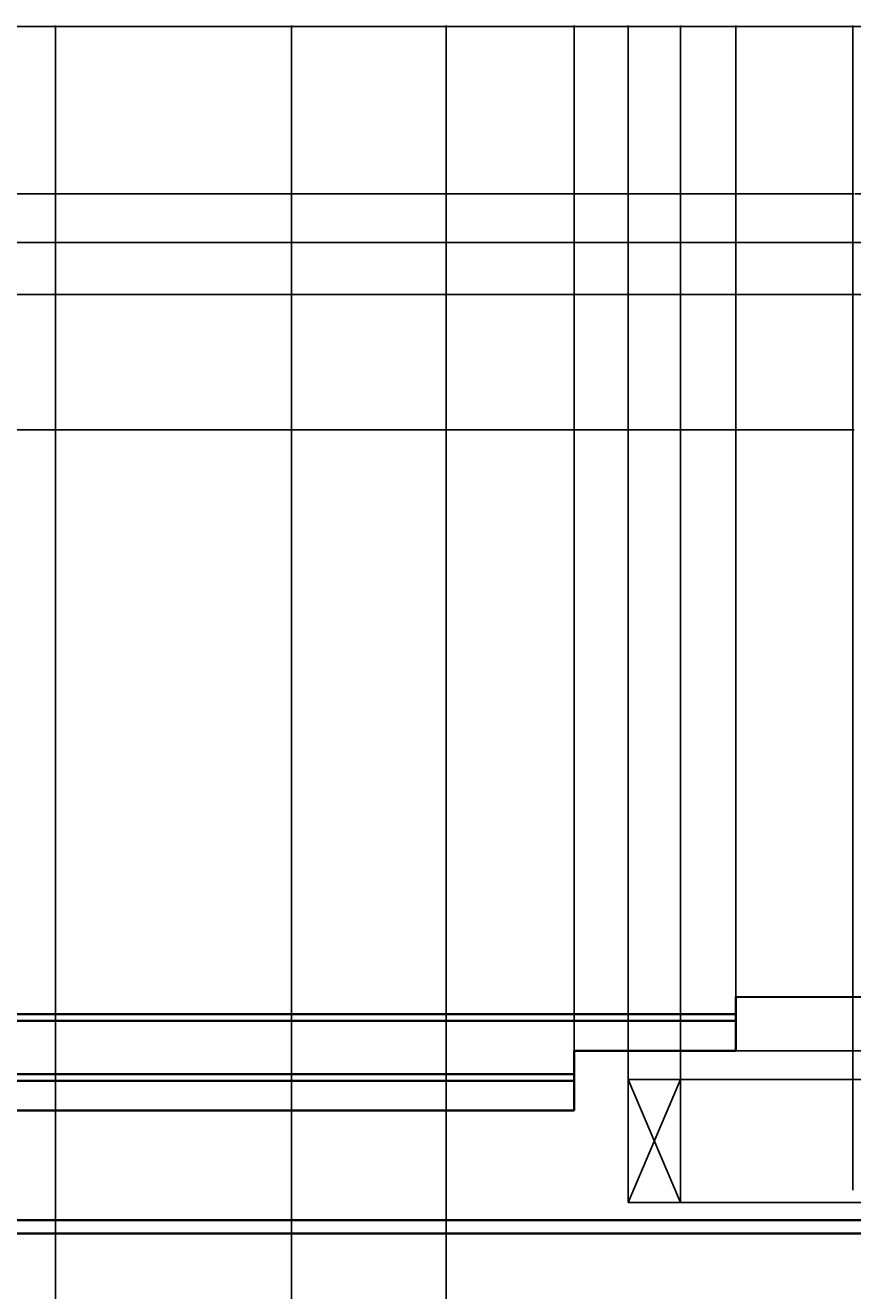
# Model space of a CAD drawing. Units: inches. Extents: x 93 to 565, y 123 to 656.
# Tile 13 of 18: x 291 to 418, y 463 to 656. Entities that reach past the tile are written whole.
import ezdxf

# ---------------------------------------------------------------- set-up
doc = ezdxf.new("R2010")
doc.units = ezdxf.units.IN
doc.header["$MEASUREMENT"] = 0
for name, color, linetype, lineweight in [('A-ANNO-DIMS', 2, 'Continuous', 18), ('A-ELEV', 7, 'Continuous', 35), ('A-GLAZ', 4, 'Continuous', 25)]:
    doc.layers.add(name, color=color, linetype=linetype, lineweight=lineweight)
doc.styles.get("Standard").update_dxf_attribs({"font": 'arial.ttf'})
doc.dimstyles.get("Standard").update_dxf_attribs({"dimtxt": 0.18, "dimasz": 0.18, "dimexe": 0.18, "dimexo": 0.0625, "dimgap": 0.09, "dimtad": 0, "dimtih": 1, "dimtoh": 1, "dimdec": 4, "dimzin": 0, "dimdsep": 46, "dimtxsty": 'Standard', "dimcen": 0.09, "dimadec": 0, "dimazin": 0, "dimtfac": 1, "dimtdec": 4, "dimtofl": 0, "dimtmove": 0, "dimatfit": 3, "dimfxl": 1, "dimtolj": 1, "dimtzin": 0, "dimarcsym": 0})

# ---------------------------------------------------------------- blocks, each defined once
blk = doc.blocks.new('*U9')
for p, q in [((0, 0), (38, 89)), ((38, 0), (0, 89))]:
    blk.add_line(p, q)
blk.add_lwpolyline([(0, 0), (38, 0), (38, 89), (0, 89)], close=True)
blk = doc.blocks.new('*D26')
at = {"layer": 'A-ANNO-DIMS', "color": 0, "lineweight": -2, "transparency": 16777216}
for p, q in [((119.08, 519.16), (119.08, 656.13)), ((119.26, 655.95), (328.79, 655.95)), ((538.9, 655.95), (329.37, 655.95)), ((539.08, 630.47), (539.08, 656.13))]:
    blk.add_line(p, q, dxfattribs=at)
at = {"layer": 'A-ANNO-DIMS', "color": 0, "transparency": 16777216}
for points in [[(119.26, 655.98), (119.26, 655.92), (119.08, 655.95)], [(538.9, 655.98), (538.9, 655.92), (539.08, 655.95)]]:
    blk.add_solid(points, dxfattribs=at)
at = {"layer": 'Defpoints', "color": 0, "transparency": 16777216}
for p in [(539.08, 655.95), (539.08, 630.4), (119.08, 519.1)]:
    blk.add_point(p, dxfattribs=at)
at = {"layer": 'A-ANNO-DIMS', "color": 0, "transparency": 16777216, "insert": (329.08, 655.95), "char_height": 0.18, "attachment_point": 5}
blk.add_mtext('\\A1;420', dxfattribs=at)
blk = doc.blocks.new('*D28')
at = {"layer": 'A-ANNO-DIMS', "color": 0, "lineweight": -2, "transparency": 16777216}
for p, q in [((210.54, 519.04), (210.54, 134)), ((295.69, 183.67), (295.69, 134)), ((210.72, 134.18), (252.72, 134.18)), ((295.51, 134.18), (253.51, 134.18))]:
    blk.add_line(p, q, dxfattribs=at)
at = {"layer": 'A-ANNO-DIMS', "color": 0, "transparency": 16777216}
for points in [[(210.72, 134.21), (210.72, 134.15), (210.54, 134.18)], [(295.51, 134.21), (295.51, 134.15), (295.69, 134.18)]]:
    blk.add_solid(points, dxfattribs=at)
at = {"layer": 'Defpoints', "color": 0, "transparency": 16777216}
for p in [(210.54, 519.1), (295.69, 183.73), (295.69, 134.18)]:
    blk.add_point(p, dxfattribs=at)
at = {"layer": 'A-ANNO-DIMS', "color": 0, "transparency": 16777216, "insert": (253.12, 134.18), "char_height": 0.18, "attachment_point": 5}
blk.add_mtext('\\A1;85.14', dxfattribs=at)
blk = doc.blocks.new('*D29')
at = {"layer": 'A-ANNO-DIMS', "color": 0, "lineweight": -2, "transparency": 16777216}
for p, q in [((437.19, 594.34), (437.19, 134)), ((295.69, 183.67), (295.69, 134)), ((295.87, 134.18), (366.05, 134.18)), ((437.01, 134.18), (366.82, 134.18))]:
    blk.add_line(p, q, dxfattribs=at)
at = {"layer": 'A-ANNO-DIMS', "color": 0, "transparency": 16777216}
for points in [[(295.87, 134.21), (295.87, 134.15), (295.69, 134.18)], [(437.01, 134.21), (437.01, 134.15), (437.19, 134.18)]]:
    blk.add_solid(points, dxfattribs=at)
at = {"layer": 'Defpoints', "color": 0, "transparency": 16777216}
for p in [(437.19, 594.4), (295.69, 183.73), (437.19, 134.18)]:
    blk.add_point(p, dxfattribs=at)
at = {"layer": 'A-ANNO-DIMS', "color": 0, "transparency": 16777216, "insert": (366.44, 134.18), "char_height": 0.18, "attachment_point": 5}
blk.add_mtext('\\A1;141.5', dxfattribs=at)
blk = doc.blocks.new('*D31')
at = {"layer": 'A-ANNO-DIMS', "color": 0, "lineweight": -2, "transparency": 16777216}
for p, q in [((417.87, 630.4), (564.81, 630.4)), ((564.63, 630.22), (564.63, 395.25)), ((564.63, 159.91), (564.63, 394.89)), ((119.14, 159.73), (564.81, 159.73))]:
    blk.add_line(p, q, dxfattribs=at)
at = {"layer": 'A-ANNO-DIMS', "color": 0, "transparency": 16777216}
for points in [[(564.6, 630.22), (564.66, 630.22), (564.63, 630.4)], [(564.6, 159.91), (564.66, 159.91), (564.63, 159.73)]]:
    blk.add_solid(points, dxfattribs=at)
at = {"layer": 'Defpoints', "color": 0, "transparency": 16777216}
for p in [(417.81, 630.4), (564.63, 630.4), (119.08, 159.73)]:
    blk.add_point(p, dxfattribs=at)
at = {"layer": 'A-ANNO-DIMS', "color": 0, "transparency": 16777216, "insert": (564.63, 395.07), "char_height": 0.18, "attachment_point": 5}
blk.add_mtext('\\A1;470.7', dxfattribs=at)
blk = doc.blocks.new('*D36')
at = {"layer": 'A-ANNO-DIMS', "color": 0, "lineweight": -2, "transparency": 16777216}
for p, q in [((417.75, 594.4), (93.35, 594.4)), ((93.53, 594.22), (93.53, 556.93)), ((93.53, 519.28), (93.53, 556.57)), ((119.02, 519.1), (93.35, 519.1))]:
    blk.add_line(p, q, dxfattribs=at)
at = {"layer": 'A-ANNO-DIMS', "color": 0, "transparency": 16777216}
for points in [[(93.5, 594.22), (93.56, 594.22), (93.53, 594.4)], [(93.5, 519.28), (93.56, 519.28), (93.53, 519.1)]]:
    blk.add_solid(points, dxfattribs=at)
at = {"layer": 'Defpoints', "color": 0, "transparency": 16777216}
for p in [(93.53, 594.4), (417.81, 594.4), (119.08, 519.1)]:
    blk.add_point(p, dxfattribs=at)
at = {"layer": 'A-ANNO-DIMS', "color": 0, "transparency": 16777216, "insert": (93.53, 556.75), "char_height": 0.18, "attachment_point": 5}
blk.add_mtext('\\A1;75.3', dxfattribs=at)
blk = doc.blocks.new('*D66')
at = {"layer": 'A-ANNO-DIMS', "color": 0, "lineweight": -2, "transparency": 16777216}
for p, q in [((295.81, 420.63), (295.81, 656.13)), ((295.99, 655.95), (313.59, 655.95)), ((331.63, 655.95), (314.03, 655.95)), ((331.81, 420.63), (331.81, 656.13))]:
    blk.add_line(p, q, dxfattribs=at)
at = {"layer": 'A-ANNO-DIMS', "color": 0, "transparency": 16777216}
for points in [[(295.99, 655.98), (295.99, 655.92), (295.81, 655.95)], [(331.63, 655.98), (331.63, 655.92), (331.81, 655.95)]]:
    blk.add_solid(points, dxfattribs=at)
at = {"layer": 'Defpoints', "color": 0, "transparency": 16777216}
for p in [(331.81, 655.95), (295.81, 420.57), (331.81, 420.57)]:
    blk.add_point(p, dxfattribs=at)
at = {"layer": 'A-ANNO-DIMS', "color": 0, "transparency": 16777216, "insert": (313.81, 655.95), "char_height": 0.18, "attachment_point": 5}
blk.add_mtext('\\A1;36', dxfattribs=at)
blk = doc.blocks.new('*D68')
at = {"layer": 'A-ANNO-DIMS', "color": 0, "lineweight": -2, "transparency": 16777216}
for p, q in [((331.81, 420.63), (331.81, 656.13)), ((331.99, 655.95), (343.24, 655.95)), ((355.28, 655.95), (344.03, 655.95)), ((355.46, 420.63), (355.46, 656.13))]:
    blk.add_line(p, q, dxfattribs=at)
at = {"layer": 'A-ANNO-DIMS', "color": 0, "transparency": 16777216}
for points in [[(331.99, 655.98), (331.99, 655.92), (331.81, 655.95)], [(355.28, 655.98), (355.28, 655.92), (355.46, 655.95)]]:
    blk.add_solid(points, dxfattribs=at)
at = {"layer": 'Defpoints', "color": 0, "transparency": 16777216}
for p in [(355.46, 655.95), (331.81, 420.57), (355.46, 420.57)]:
    blk.add_point(p, dxfattribs=at)
at = {"layer": 'A-ANNO-DIMS', "color": 0, "transparency": 16777216, "insert": (343.64, 655.95), "char_height": 0.18, "attachment_point": 5}
blk.add_mtext('\\A1;23.65', dxfattribs=at)
blk = doc.blocks.new('*D69')
at = {"layer": 'A-ANNO-DIMS', "color": 0, "lineweight": -2, "transparency": 16777216}
for p, q in [((355.46, 420.63), (355.46, 656.13)), ((355.64, 655.95), (391.65, 655.95)), ((428.44, 655.95), (392.43, 655.95)), ((428.62, 420.63), (428.62, 656.13))]:
    blk.add_line(p, q, dxfattribs=at)
at = {"layer": 'A-ANNO-DIMS', "color": 0, "transparency": 16777216}
for points in [[(355.64, 655.98), (355.64, 655.92), (355.46, 655.95)], [(428.44, 655.98), (428.44, 655.92), (428.62, 655.95)]]:
    blk.add_solid(points, dxfattribs=at)
at = {"layer": 'Defpoints', "color": 0, "transparency": 16777216}
for p in [(428.62, 655.95), (355.46, 420.57), (428.62, 420.57)]:
    blk.add_point(p, dxfattribs=at)
at = {"layer": 'A-ANNO-DIMS', "color": 0, "transparency": 16777216, "insert": (392.04, 655.95), "char_height": 0.18, "attachment_point": 5}
blk.add_mtext('\\A1;73.16', dxfattribs=at)
blk = doc.blocks.new('*D75')
at = {"layer": 'A-ANNO-DIMS', "color": 0, "lineweight": -2, "transparency": 16777216}
for p, q in [((375.01, 499.67), (375.01, 656.13)), ((375.19, 655.95), (386.89, 655.95)), ((399.51, 655.95), (387.82, 655.95)), ((399.69, 507.89), (399.69, 656.13))]:
    blk.add_line(p, q, dxfattribs=at)
at = {"layer": 'A-ANNO-DIMS', "color": 0, "transparency": 16777216}
for points in [[(375.19, 655.98), (375.19, 655.92), (375.01, 655.95)], [(399.51, 655.98), (399.51, 655.92), (399.69, 655.95)]]:
    blk.add_solid(points, dxfattribs=at)
at = {"layer": 'Defpoints', "color": 0, "transparency": 16777216}
for p in [(399.69, 655.95), (399.69, 507.83), (375.01, 499.61)]:
    blk.add_point(p, dxfattribs=at)
at = {"layer": 'A-ANNO-DIMS', "color": 0, "transparency": 16777216, "insert": (387.35, 655.95), "char_height": 0.18, "attachment_point": 5}
blk.add_mtext('\\A1;24.683', dxfattribs=at)
blk = doc.blocks.new('*D76')
at = {"layer": 'A-ANNO-DIMS', "color": 0, "lineweight": -2, "transparency": 16777216}
for p, q in [((399.69, 507.89), (399.69, 656.13)), ((399.87, 655.95), (417.98, 655.95)), ((437.01, 655.95), (418.9, 655.95)), ((437.19, 507.79), (437.19, 656.13))]:
    blk.add_line(p, q, dxfattribs=at)
at = {"layer": 'A-ANNO-DIMS', "color": 0, "transparency": 16777216}
for points in [[(399.87, 655.98), (399.87, 655.92), (399.69, 655.95)], [(437.01, 655.98), (437.01, 655.92), (437.19, 655.95)]]:
    blk.add_solid(points, dxfattribs=at)
at = {"layer": 'Defpoints', "color": 0, "transparency": 16777216}
for p in [(437.19, 655.95), (399.69, 507.83), (437.19, 507.73)]:
    blk.add_point(p, dxfattribs=at)
at = {"layer": 'A-ANNO-DIMS', "color": 0, "transparency": 16777216, "insert": (418.44, 655.95), "char_height": 0.18, "attachment_point": 5}
blk.add_mtext('\\A1;37.494', dxfattribs=at)
blk = doc.blocks.new('*D77')
at = {"layer": 'A-ANNO-DIMS', "color": 0, "lineweight": -2, "transparency": 16777216}
for p, q in [((399.76, 507.83), (564.81, 507.83)), ((564.63, 507.65), (564.63, 503.9)), ((564.63, 499.79), (564.63, 503.54)), ((375.07, 499.61), (564.81, 499.61))]:
    blk.add_line(p, q, dxfattribs=at)
at = {"layer": 'A-ANNO-DIMS', "color": 0, "transparency": 16777216}
for points in [[(564.6, 507.65), (564.66, 507.65), (564.63, 507.83)], [(564.6, 499.79), (564.66, 499.79), (564.63, 499.61)]]:
    blk.add_solid(points, dxfattribs=at)
at = {"layer": 'Defpoints', "color": 0, "transparency": 16777216}
for p in [(399.69, 507.83), (564.63, 507.83), (375.01, 499.61)]:
    blk.add_point(p, dxfattribs=at)
at = {"layer": 'A-ANNO-DIMS', "color": 0, "transparency": 16777216, "insert": (564.63, 503.72), "char_height": 0.18, "attachment_point": 5}
blk.add_mtext('\\A1;8.221', dxfattribs=at)
blk = doc.blocks.new('*D78')
at = {"layer": 'A-ANNO-DIMS', "color": 0, "lineweight": -2, "transparency": 16777216}
for p, q in [((383.21, 495.28), (383.21, 656.13)), ((383.39, 655.95), (386.82, 655.95)), ((391.04, 655.95), (387.61, 655.95)), ((391.22, 495.28), (391.22, 656.13))]:
    blk.add_line(p, q, dxfattribs=at)
at = {"layer": 'A-ANNO-DIMS', "color": 0, "transparency": 16777216}
for points in [[(383.39, 655.98), (383.39, 655.92), (383.21, 655.95)], [(391.04, 655.98), (391.04, 655.92), (391.22, 655.95)]]:
    blk.add_solid(points, dxfattribs=at)
at = {"layer": 'Defpoints', "color": 0, "transparency": 16777216}
for p in [(391.22, 655.95), (383.21, 495.22), (391.22, 495.22)]:
    blk.add_point(p, dxfattribs=at)
at = {"layer": 'A-ANNO-DIMS', "color": 0, "transparency": 16777216, "insert": (387.22, 655.95), "char_height": 0.18, "attachment_point": 5}
blk.add_mtext('\\A1;8.007', dxfattribs=at)
blk = doc.blocks.new('*D79')
at = {"layer": 'A-ANNO-DIMS', "color": 0, "lineweight": -2, "transparency": 16777216}
for p, q in [((391.28, 495.22), (564.81, 495.22)), ((564.63, 495.04), (564.63, 486.02)), ((564.63, 476.64), (564.63, 485.66)), ((391.28, 476.46), (564.81, 476.46))]:
    blk.add_line(p, q, dxfattribs=at)
at = {"layer": 'A-ANNO-DIMS', "color": 0, "transparency": 16777216}
for points in [[(564.6, 495.04), (564.66, 495.04), (564.63, 495.22)], [(564.6, 476.64), (564.66, 476.64), (564.63, 476.46)]]:
    blk.add_solid(points, dxfattribs=at)
at = {"layer": 'Defpoints', "color": 0, "transparency": 16777216}
for p in [(391.22, 495.22), (564.63, 495.22), (391.22, 476.46)]:
    blk.add_point(p, dxfattribs=at)
at = {"layer": 'A-ANNO-DIMS', "color": 0, "transparency": 16777216, "insert": (564.63, 485.84), "char_height": 0.18, "attachment_point": 5}
blk.add_mtext('\\A1;18.753', dxfattribs=at)
blk = doc.blocks.new('*D80')
at = {"layer": 'A-ANNO-DIMS', "color": 0, "lineweight": -2, "transparency": 16777216}
for p, q in [((375.01, 499.67), (375.01, 656.13)), ((375.19, 655.95), (378.72, 655.95)), ((383.03, 655.95), (379.51, 655.95)), ((383.21, 495.28), (383.21, 656.13))]:
    blk.add_line(p, q, dxfattribs=at)
at = {"layer": 'A-ANNO-DIMS', "color": 0, "transparency": 16777216}
for points in [[(375.19, 655.98), (375.19, 655.92), (375.01, 655.95)], [(383.03, 655.98), (383.03, 655.92), (383.21, 655.95)]]:
    blk.add_solid(points, dxfattribs=at)
at = {"layer": 'Defpoints', "color": 0, "transparency": 16777216}
for p in [(383.21, 655.95), (375.01, 499.61), (383.21, 495.22)]:
    blk.add_point(p, dxfattribs=at)
at = {"layer": 'A-ANNO-DIMS', "color": 0, "transparency": 16777216, "insert": (379.11, 655.95), "char_height": 0.18, "attachment_point": 5}
blk.add_mtext('\\A1;8.203', dxfattribs=at)
blk = doc.blocks.new('*D81')
at = {"layer": 'A-ANNO-DIMS', "color": 0, "lineweight": -2, "transparency": 16777216}
for p, q in [((391.22, 476.53), (391.22, 656.13)), ((391.4, 655.95), (403.97, 655.95)), ((417.33, 655.95), (404.76, 655.95)), ((417.51, 478.33), (417.51, 656.13))]:
    blk.add_line(p, q, dxfattribs=at)
at = {"layer": 'A-ANNO-DIMS', "color": 0, "transparency": 16777216}
for points in [[(391.4, 655.98), (391.4, 655.92), (391.22, 655.95)], [(417.33, 655.98), (417.33, 655.92), (417.51, 655.95)]]:
    blk.add_solid(points, dxfattribs=at)
at = {"layer": 'Defpoints', "color": 0, "transparency": 16777216}
for p in [(417.51, 655.95), (417.51, 478.26), (391.22, 476.46)]:
    blk.add_point(p, dxfattribs=at)
at = {"layer": 'A-ANNO-DIMS', "color": 0, "transparency": 16777216, "insert": (404.37, 655.95), "char_height": 0.18, "attachment_point": 5}
blk.add_mtext('\\A1;26.29', dxfattribs=at)
blk = doc.blocks.new('*D94')
at = {"layer": 'A-ANNO-DIMS', "color": 0, "lineweight": -2, "transparency": 16777216}
for p, q in [((423.75, 615.04), (93.35, 615.04)), ((93.53, 614.86), (93.53, 604.9)), ((93.53, 594.58), (93.53, 604.54)), ((417.75, 594.4), (93.35, 594.4))]:
    blk.add_line(p, q, dxfattribs=at)
at = {"layer": 'A-ANNO-DIMS', "color": 0, "transparency": 16777216}
for points in [[(93.5, 614.86), (93.56, 614.86), (93.53, 615.04)], [(93.5, 594.58), (93.56, 594.58), (93.53, 594.4)]]:
    blk.add_solid(points, dxfattribs=at)
at = {"layer": 'Defpoints', "color": 0, "transparency": 16777216}
for p in [(93.53, 615.04), (423.81, 615.04), (417.81, 594.4)]:
    blk.add_point(p, dxfattribs=at)
at = {"layer": 'A-ANNO-DIMS', "color": 0, "transparency": 16777216, "insert": (93.53, 604.72), "char_height": 0.18, "attachment_point": 5}
blk.add_mtext('\\A1;20.636', dxfattribs=at)
blk = doc.blocks.new('*D95')
at = {"layer": 'A-ANNO-DIMS', "color": 0, "lineweight": -2, "transparency": 16777216}
for p, q in [((487.73, 622.97), (93.35, 622.97)), ((93.53, 622.79), (93.53, 619.19)), ((93.53, 615.22), (93.53, 618.82)), ((423.75, 615.04), (93.35, 615.04))]:
    blk.add_line(p, q, dxfattribs=at)
at = {"layer": 'A-ANNO-DIMS', "color": 0, "transparency": 16777216}
for points in [[(93.5, 622.79), (93.56, 622.79), (93.53, 622.97)], [(93.5, 615.22), (93.56, 615.22), (93.53, 615.04)]]:
    blk.add_solid(points, dxfattribs=at)
at = {"layer": 'Defpoints', "color": 0, "transparency": 16777216}
for p in [(93.53, 622.97), (487.8, 622.97), (423.81, 615.04)]:
    blk.add_point(p, dxfattribs=at)
at = {"layer": 'A-ANNO-DIMS', "color": 0, "transparency": 16777216, "insert": (93.53, 619.01), "char_height": 0.18, "attachment_point": 5}
blk.add_mtext('\\A1;7.93', dxfattribs=at)
blk = doc.blocks.new('*D96')
at = {"layer": 'A-ANNO-DIMS', "color": 0, "lineweight": -2, "transparency": 16777216}
for p, q in [((417.75, 630.4), (93.35, 630.4)), ((93.53, 630.22), (93.53, 626.87)), ((93.53, 623.15), (93.53, 626.51)), ((487.73, 622.97), (93.35, 622.97))]:
    blk.add_line(p, q, dxfattribs=at)
at = {"layer": 'A-ANNO-DIMS', "color": 0, "transparency": 16777216}
for points in [[(93.5, 630.22), (93.56, 630.22), (93.53, 630.4)], [(93.5, 623.15), (93.56, 623.15), (93.53, 622.97)]]:
    blk.add_solid(points, dxfattribs=at)
at = {"layer": 'Defpoints', "color": 0, "transparency": 16777216}
for p in [(93.53, 630.4), (417.81, 630.4), (487.8, 622.97)]:
    blk.add_point(p, dxfattribs=at)
at = {"layer": 'A-ANNO-DIMS', "color": 0, "transparency": 16777216, "insert": (93.53, 626.69), "char_height": 0.18, "attachment_point": 5}
blk.add_mtext('\\A1;7.434', dxfattribs=at)
blk = doc.blocks.new('*D105')
at = {"layer": 'A-ANNO-DIMS', "color": 0, "lineweight": -2, "transparency": 16777216}
for p, q in [((119.08, 519.16), (119.08, 656.13)), ((119.26, 655.95), (328.54, 655.95)), ((538.9, 655.95), (329.62, 655.95)), ((539.08, 630.47), (539.08, 656.13))]:
    blk.add_line(p, q, dxfattribs=at)
at = {"layer": 'A-ANNO-DIMS', "color": 0, "transparency": 16777216}
for points in [[(119.26, 655.98), (119.26, 655.92), (119.08, 655.95)], [(538.9, 655.98), (538.9, 655.92), (539.08, 655.95)]]:
    blk.add_solid(points, dxfattribs=at)
at = {"layer": 'Defpoints', "color": 0, "transparency": 16777216}
for p in [(539.08, 655.95), (539.08, 630.4), (119.08, 519.1)]:
    blk.add_point(p, dxfattribs=at)
at = {"layer": 'A-ANNO-DIMS', "color": 0, "transparency": 16777216, "insert": (329.08, 655.95), "char_height": 0.18, "attachment_point": 5}
blk.add_mtext('\\A1;420.000', dxfattribs=at)
blk = doc.blocks.new('*D107')
at = {"layer": 'A-ANNO-DIMS', "color": 0, "lineweight": -2, "transparency": 16777216}
for p, q in [((210.54, 519.04), (210.54, 134)), ((295.69, 183.67), (295.69, 134)), ((210.72, 134.18), (252.65, 134.18)), ((295.51, 134.18), (253.58, 134.18))]:
    blk.add_line(p, q, dxfattribs=at)
at = {"layer": 'A-ANNO-DIMS', "color": 0, "transparency": 16777216}
for points in [[(210.72, 134.21), (210.72, 134.15), (210.54, 134.18)], [(295.51, 134.21), (295.51, 134.15), (295.69, 134.18)]]:
    blk.add_solid(points, dxfattribs=at)
at = {"layer": 'Defpoints', "color": 0, "transparency": 16777216}
for p in [(210.54, 519.1), (295.69, 183.73), (295.69, 134.18)]:
    blk.add_point(p, dxfattribs=at)
at = {"layer": 'A-ANNO-DIMS', "color": 0, "transparency": 16777216, "insert": (253.12, 134.18), "char_height": 0.18, "attachment_point": 5}
blk.add_mtext('\\A1;85.143', dxfattribs=at)
blk = doc.blocks.new('*D108')
at = {"layer": 'A-ANNO-DIMS', "color": 0, "lineweight": -2, "transparency": 16777216}
for p, q in [((437.19, 594.34), (437.19, 134)), ((295.69, 183.67), (295.69, 134)), ((295.87, 134.18), (365.93, 134.18)), ((437.01, 134.18), (366.95, 134.18))]:
    blk.add_line(p, q, dxfattribs=at)
at = {"layer": 'A-ANNO-DIMS', "color": 0, "transparency": 16777216}
for points in [[(295.87, 134.21), (295.87, 134.15), (295.69, 134.18)], [(437.01, 134.21), (437.01, 134.15), (437.19, 134.18)]]:
    blk.add_solid(points, dxfattribs=at)
at = {"layer": 'Defpoints', "color": 0, "transparency": 16777216}
for p in [(437.19, 594.4), (295.69, 183.73), (437.19, 134.18)]:
    blk.add_point(p, dxfattribs=at)
at = {"layer": 'A-ANNO-DIMS', "color": 0, "transparency": 16777216, "insert": (366.44, 134.18), "char_height": 0.18, "attachment_point": 5}
blk.add_mtext('\\A1;141.501', dxfattribs=at)
blk = doc.blocks.new('*D110')
at = {"layer": 'A-ANNO-DIMS', "color": 0, "lineweight": -2, "transparency": 16777216}
for p, q in [((417.87, 630.4), (564.81, 630.4)), ((564.63, 630.22), (564.63, 395.25)), ((564.63, 159.91), (564.63, 394.89)), ((119.14, 159.73), (564.81, 159.73))]:
    blk.add_line(p, q, dxfattribs=at)
at = {"layer": 'A-ANNO-DIMS', "color": 0, "transparency": 16777216}
for points in [[(564.6, 630.22), (564.66, 630.22), (564.63, 630.4)], [(564.6, 159.91), (564.66, 159.91), (564.63, 159.73)]]:
    blk.add_solid(points, dxfattribs=at)
at = {"layer": 'Defpoints', "color": 0, "transparency": 16777216}
for p in [(417.81, 630.4), (564.63, 630.4), (119.08, 159.73)]:
    blk.add_point(p, dxfattribs=at)
at = {"layer": 'A-ANNO-DIMS', "color": 0, "transparency": 16777216, "insert": (564.63, 395.07), "char_height": 0.18, "attachment_point": 5}
blk.add_mtext('\\A1;470.673', dxfattribs=at)
blk = doc.blocks.new('*D115')
at = {"layer": 'A-ANNO-DIMS', "color": 0, "lineweight": -2, "transparency": 16777216}
for p, q in [((417.75, 594.4), (93.35, 594.4)), ((93.53, 594.22), (93.53, 556.93)), ((93.53, 519.28), (93.53, 556.57)), ((119.02, 519.1), (93.35, 519.1))]:
    blk.add_line(p, q, dxfattribs=at)
at = {"layer": 'A-ANNO-DIMS', "color": 0, "transparency": 16777216}
for points in [[(93.5, 594.22), (93.56, 594.22), (93.53, 594.4)], [(93.5, 519.28), (93.56, 519.28), (93.53, 519.1)]]:
    blk.add_solid(points, dxfattribs=at)
at = {"layer": 'Defpoints', "color": 0, "transparency": 16777216}
for p in [(93.53, 594.4), (417.81, 594.4), (119.08, 519.1)]:
    blk.add_point(p, dxfattribs=at)
at = {"layer": 'A-ANNO-DIMS', "color": 0, "transparency": 16777216, "insert": (93.53, 556.75), "char_height": 0.18, "attachment_point": 5}
blk.add_mtext('\\A1;75.305', dxfattribs=at)
blk = doc.blocks.new('*D145')
at = {"layer": 'A-ANNO-DIMS', "color": 0, "lineweight": -2, "transparency": 16777216}
for p, q in [((295.81, 420.63), (295.81, 656.13)), ((295.99, 655.95), (313.35, 655.95)), ((331.63, 655.95), (314.27, 655.95)), ((331.81, 420.63), (331.81, 656.13))]:
    blk.add_line(p, q, dxfattribs=at)
at = {"layer": 'A-ANNO-DIMS', "color": 0, "transparency": 16777216}
for points in [[(295.99, 655.98), (295.99, 655.92), (295.81, 655.95)], [(331.63, 655.98), (331.63, 655.92), (331.81, 655.95)]]:
    blk.add_solid(points, dxfattribs=at)
at = {"layer": 'Defpoints', "color": 0, "transparency": 16777216}
for p in [(331.81, 655.95), (295.81, 420.57), (331.81, 420.57)]:
    blk.add_point(p, dxfattribs=at)
at = {"layer": 'A-ANNO-DIMS', "color": 0, "transparency": 16777216, "insert": (313.81, 655.95), "char_height": 0.18, "attachment_point": 5}
blk.add_mtext('\\A1;36.000', dxfattribs=at)
blk = doc.blocks.new('*D147')
at = {"layer": 'A-ANNO-DIMS', "color": 0, "lineweight": -2, "transparency": 16777216}
for p, q in [((331.81, 420.63), (331.81, 656.13)), ((331.99, 655.95), (343.17, 655.95)), ((355.28, 655.95), (344.1, 655.95)), ((355.46, 420.63), (355.46, 656.13))]:
    blk.add_line(p, q, dxfattribs=at)
at = {"layer": 'A-ANNO-DIMS', "color": 0, "transparency": 16777216}
for points in [[(331.99, 655.98), (331.99, 655.92), (331.81, 655.95)], [(355.28, 655.98), (355.28, 655.92), (355.46, 655.95)]]:
    blk.add_solid(points, dxfattribs=at)
at = {"layer": 'Defpoints', "color": 0, "transparency": 16777216}
for p in [(355.46, 655.95), (331.81, 420.57), (355.46, 420.57)]:
    blk.add_point(p, dxfattribs=at)
at = {"layer": 'A-ANNO-DIMS', "color": 0, "transparency": 16777216, "insert": (343.64, 655.95), "char_height": 0.18, "attachment_point": 5}
blk.add_mtext('\\A1;23.649', dxfattribs=at)
blk = doc.blocks.new('*D148')
at = {"layer": 'A-ANNO-DIMS', "color": 0, "lineweight": -2, "transparency": 16777216}
for p, q in [((355.46, 420.63), (355.46, 656.13)), ((355.64, 655.95), (391.58, 655.95)), ((428.44, 655.95), (392.5, 655.95)), ((428.62, 420.63), (428.62, 656.13))]:
    blk.add_line(p, q, dxfattribs=at)
at = {"layer": 'A-ANNO-DIMS', "color": 0, "transparency": 16777216}
for points in [[(355.64, 655.98), (355.64, 655.92), (355.46, 655.95)], [(428.44, 655.98), (428.44, 655.92), (428.62, 655.95)]]:
    blk.add_solid(points, dxfattribs=at)
at = {"layer": 'Defpoints', "color": 0, "transparency": 16777216}
for p in [(428.62, 655.95), (355.46, 420.57), (428.62, 420.57)]:
    blk.add_point(p, dxfattribs=at)
at = {"layer": 'A-ANNO-DIMS', "color": 0, "transparency": 16777216, "insert": (392.04, 655.95), "char_height": 0.18, "attachment_point": 5}
blk.add_mtext('\\A1;73.156', dxfattribs=at)
blk = doc.blocks.new('*D154')
at = {"layer": 'A-ANNO-DIMS', "color": 0, "lineweight": -2, "transparency": 16777216}
for p, q in [((375.01, 499.67), (375.01, 656.13)), ((375.19, 655.95), (386.89, 655.95)), ((399.51, 655.95), (387.82, 655.95)), ((399.69, 507.89), (399.69, 656.13))]:
    blk.add_line(p, q, dxfattribs=at)
at = {"layer": 'A-ANNO-DIMS', "color": 0, "transparency": 16777216}
for points in [[(375.19, 655.98), (375.19, 655.92), (375.01, 655.95)], [(399.51, 655.98), (399.51, 655.92), (399.69, 655.95)]]:
    blk.add_solid(points, dxfattribs=at)
at = {"layer": 'Defpoints', "color": 0, "transparency": 16777216}
for p in [(399.69, 655.95), (399.69, 507.83), (375.01, 499.61)]:
    blk.add_point(p, dxfattribs=at)
at = {"layer": 'A-ANNO-DIMS', "color": 0, "transparency": 16777216, "insert": (387.35, 655.95), "char_height": 0.18, "attachment_point": 5}
blk.add_mtext('\\A1;24.683', dxfattribs=at)
blk = doc.blocks.new('*D155')
at = {"layer": 'A-ANNO-DIMS', "color": 0, "lineweight": -2, "transparency": 16777216}
for p, q in [((399.69, 507.89), (399.69, 656.13)), ((399.87, 655.95), (417.98, 655.95)), ((437.01, 655.95), (418.9, 655.95)), ((437.19, 507.79), (437.19, 656.13))]:
    blk.add_line(p, q, dxfattribs=at)
at = {"layer": 'A-ANNO-DIMS', "color": 0, "transparency": 16777216}
for points in [[(399.87, 655.98), (399.87, 655.92), (399.69, 655.95)], [(437.01, 655.98), (437.01, 655.92), (437.19, 655.95)]]:
    blk.add_solid(points, dxfattribs=at)
at = {"layer": 'Defpoints', "color": 0, "transparency": 16777216}
for p in [(437.19, 655.95), (399.69, 507.83), (437.19, 507.73)]:
    blk.add_point(p, dxfattribs=at)
at = {"layer": 'A-ANNO-DIMS', "color": 0, "transparency": 16777216, "insert": (418.44, 655.95), "char_height": 0.18, "attachment_point": 5}
blk.add_mtext('\\A1;37.494', dxfattribs=at)
blk = doc.blocks.new('*D156')
at = {"layer": 'A-ANNO-DIMS', "color": 0, "lineweight": -2, "transparency": 16777216}
for p, q in [((399.76, 507.83), (564.81, 507.83)), ((564.63, 507.65), (564.63, 503.9)), ((564.63, 499.79), (564.63, 503.54)), ((375.07, 499.61), (564.81, 499.61))]:
    blk.add_line(p, q, dxfattribs=at)
at = {"layer": 'A-ANNO-DIMS', "color": 0, "transparency": 16777216}
for points in [[(564.6, 507.65), (564.66, 507.65), (564.63, 507.83)], [(564.6, 499.79), (564.66, 499.79), (564.63, 499.61)]]:
    blk.add_solid(points, dxfattribs=at)
at = {"layer": 'Defpoints', "color": 0, "transparency": 16777216}
for p in [(399.69, 507.83), (564.63, 507.83), (375.01, 499.61)]:
    blk.add_point(p, dxfattribs=at)
at = {"layer": 'A-ANNO-DIMS', "color": 0, "transparency": 16777216, "insert": (564.63, 503.72), "char_height": 0.18, "attachment_point": 5}
blk.add_mtext('\\A1;8.221', dxfattribs=at)
blk = doc.blocks.new('*D157')
at = {"layer": 'A-ANNO-DIMS', "color": 0, "lineweight": -2, "transparency": 16777216}
for p, q in [((383.21, 495.28), (383.21, 656.13)), ((383.39, 655.95), (386.82, 655.95)), ((391.04, 655.95), (387.61, 655.95)), ((391.22, 495.28), (391.22, 656.13))]:
    blk.add_line(p, q, dxfattribs=at)
at = {"layer": 'A-ANNO-DIMS', "color": 0, "transparency": 16777216}
for points in [[(383.39, 655.98), (383.39, 655.92), (383.21, 655.95)], [(391.04, 655.98), (391.04, 655.92), (391.22, 655.95)]]:
    blk.add_solid(points, dxfattribs=at)
at = {"layer": 'Defpoints', "color": 0, "transparency": 16777216}
for p in [(391.22, 655.95), (383.21, 495.22), (391.22, 495.22)]:
    blk.add_point(p, dxfattribs=at)
at = {"layer": 'A-ANNO-DIMS', "color": 0, "transparency": 16777216, "insert": (387.22, 655.95), "char_height": 0.18, "attachment_point": 5}
blk.add_mtext('\\A1;8.007', dxfattribs=at)
blk = doc.blocks.new('*D158')
at = {"layer": 'A-ANNO-DIMS', "color": 0, "lineweight": -2, "transparency": 16777216}
for p, q in [((391.28, 495.22), (564.81, 495.22)), ((564.63, 495.04), (564.63, 486.02)), ((564.63, 476.64), (564.63, 485.66)), ((391.28, 476.46), (564.81, 476.46))]:
    blk.add_line(p, q, dxfattribs=at)
at = {"layer": 'A-ANNO-DIMS', "color": 0, "transparency": 16777216}
for points in [[(564.6, 495.04), (564.66, 495.04), (564.63, 495.22)], [(564.6, 476.64), (564.66, 476.64), (564.63, 476.46)]]:
    blk.add_solid(points, dxfattribs=at)
at = {"layer": 'Defpoints', "color": 0, "transparency": 16777216}
for p in [(391.22, 495.22), (564.63, 495.22), (391.22, 476.46)]:
    blk.add_point(p, dxfattribs=at)
at = {"layer": 'A-ANNO-DIMS', "color": 0, "transparency": 16777216, "insert": (564.63, 485.84), "char_height": 0.18, "attachment_point": 5}
blk.add_mtext('\\A1;18.753', dxfattribs=at)
blk = doc.blocks.new('*D159')
at = {"layer": 'A-ANNO-DIMS', "color": 0, "lineweight": -2, "transparency": 16777216}
for p, q in [((375.01, 499.67), (375.01, 656.13)), ((375.19, 655.95), (378.72, 655.95)), ((383.03, 655.95), (379.51, 655.95)), ((383.21, 495.28), (383.21, 656.13))]:
    blk.add_line(p, q, dxfattribs=at)
at = {"layer": 'A-ANNO-DIMS', "color": 0, "transparency": 16777216}
for points in [[(375.19, 655.98), (375.19, 655.92), (375.01, 655.95)], [(383.03, 655.98), (383.03, 655.92), (383.21, 655.95)]]:
    blk.add_solid(points, dxfattribs=at)
at = {"layer": 'Defpoints', "color": 0, "transparency": 16777216}
for p in [(383.21, 655.95), (375.01, 499.61), (383.21, 495.22)]:
    blk.add_point(p, dxfattribs=at)
at = {"layer": 'A-ANNO-DIMS', "color": 0, "transparency": 16777216, "insert": (379.11, 655.95), "char_height": 0.18, "attachment_point": 5}
blk.add_mtext('\\A1;8.203', dxfattribs=at)
blk = doc.blocks.new('*D160')
at = {"layer": 'A-ANNO-DIMS', "color": 0, "lineweight": -2, "transparency": 16777216}
for p, q in [((391.22, 476.53), (391.22, 656.13)), ((391.4, 655.95), (403.92, 655.95)), ((417.33, 655.95), (404.82, 655.95)), ((417.51, 478.33), (417.51, 656.13))]:
    blk.add_line(p, q, dxfattribs=at)
at = {"layer": 'A-ANNO-DIMS', "color": 0, "transparency": 16777216}
for points in [[(391.4, 655.98), (391.4, 655.92), (391.22, 655.95)], [(417.33, 655.98), (417.33, 655.92), (417.51, 655.95)]]:
    blk.add_solid(points, dxfattribs=at)
at = {"layer": 'Defpoints', "color": 0, "transparency": 16777216}
for p in [(417.51, 655.95), (417.51, 478.26), (391.22, 476.46)]:
    blk.add_point(p, dxfattribs=at)
at = {"layer": 'A-ANNO-DIMS', "color": 0, "transparency": 16777216, "insert": (404.37, 655.95), "char_height": 0.18, "attachment_point": 5}
blk.add_mtext('\\A1;26.291', dxfattribs=at)
blk = doc.blocks.new('*D173')
at = {"layer": 'A-ANNO-DIMS', "color": 0, "lineweight": -2, "transparency": 16777216}
for p, q in [((423.75, 615.04), (93.35, 615.04)), ((93.53, 614.86), (93.53, 604.9)), ((93.53, 594.58), (93.53, 604.54)), ((417.75, 594.4), (93.35, 594.4))]:
    blk.add_line(p, q, dxfattribs=at)
at = {"layer": 'A-ANNO-DIMS', "color": 0, "transparency": 16777216}
for points in [[(93.5, 614.86), (93.56, 614.86), (93.53, 615.04)], [(93.5, 594.58), (93.56, 594.58), (93.53, 594.4)]]:
    blk.add_solid(points, dxfattribs=at)
at = {"layer": 'Defpoints', "color": 0, "transparency": 16777216}
for p in [(93.53, 615.04), (423.81, 615.04), (417.81, 594.4)]:
    blk.add_point(p, dxfattribs=at)
at = {"layer": 'A-ANNO-DIMS', "color": 0, "transparency": 16777216, "insert": (93.53, 604.72), "char_height": 0.18, "attachment_point": 5}
blk.add_mtext('\\A1;20.636', dxfattribs=at)
blk = doc.blocks.new('*D174')
at = {"layer": 'A-ANNO-DIMS', "color": 0, "lineweight": -2, "transparency": 16777216}
for p, q in [((487.73, 622.97), (93.35, 622.97)), ((93.53, 622.79), (93.53, 619.19)), ((93.53, 615.22), (93.53, 618.82)), ((423.75, 615.04), (93.35, 615.04))]:
    blk.add_line(p, q, dxfattribs=at)
at = {"layer": 'A-ANNO-DIMS', "color": 0, "transparency": 16777216}
for points in [[(93.5, 622.79), (93.56, 622.79), (93.53, 622.97)], [(93.5, 615.22), (93.56, 615.22), (93.53, 615.04)]]:
    blk.add_solid(points, dxfattribs=at)
at = {"layer": 'Defpoints', "color": 0, "transparency": 16777216}
for p in [(93.53, 622.97), (487.8, 622.97), (423.81, 615.04)]:
    blk.add_point(p, dxfattribs=at)
at = {"layer": 'A-ANNO-DIMS', "color": 0, "transparency": 16777216, "insert": (93.53, 619.01), "char_height": 0.18, "attachment_point": 5}
blk.add_mtext('\\A1;7.930', dxfattribs=at)
blk = doc.blocks.new('*D175')
at = {"layer": 'A-ANNO-DIMS', "color": 0, "lineweight": -2, "transparency": 16777216}
for p, q in [((417.75, 630.4), (93.35, 630.4)), ((93.53, 630.22), (93.53, 626.87)), ((93.53, 623.15), (93.53, 626.51)), ((487.73, 622.97), (93.35, 622.97))]:
    blk.add_line(p, q, dxfattribs=at)
at = {"layer": 'A-ANNO-DIMS', "color": 0, "transparency": 16777216}
for points in [[(93.5, 630.22), (93.56, 630.22), (93.53, 630.4)], [(93.5, 623.15), (93.56, 623.15), (93.53, 622.97)]]:
    blk.add_solid(points, dxfattribs=at)
at = {"layer": 'Defpoints', "color": 0, "transparency": 16777216}
for p in [(93.53, 630.4), (417.81, 630.4), (487.8, 622.97)]:
    blk.add_point(p, dxfattribs=at)
at = {"layer": 'A-ANNO-DIMS', "color": 0, "transparency": 16777216, "insert": (93.53, 626.69), "char_height": 0.18, "attachment_point": 5}
blk.add_mtext('\\A1;7.434', dxfattribs=at)

msp = doc.modelspace()

# ---------------------------------------------------------------- linework, layer by layer
at = {"layer": 'A-ELEV'}
for p, q in [((399.6946, 507.8299), (437.1885, 507.7323)), ((399.6946, 507.8299), (399.6946, 499.609)), ((399.6946, 505.2018), (210.5443, 505.2018)), ((399.6946, 504.2018), (210.5443, 504.2018)), ((399.6946, 499.609), (375.0121, 499.609)), ((375.0121, 499.609), (375.0121, 490.4746)), ((375.0121, 496.0418), (210.5443, 496.0418)), ((375.0121, 495.0418), (210.5443, 495.0418)), ((375.0121, 490.4746), (210.5443, 490.4746)), ((210.5443, 473.7323), (437.1885, 473.7323)), ((210.5443, 471.7323), (437.1885, 471.7323))]:
    msp.add_line(p, q, dxfattribs=at)

# ---------------------------------------------------------------- block references
at = {"layer": 'A-GLAZ', "xscale": 0.2107133031769033, "yscale": 0.2107133031769033, "zscale": 0.2107133031769033}
msp.add_blockref('*U9', (383.2149, 476.4637), dxfattribs=at)

# ---------------------------------------------------------------- dimensions: what is measured, and where the dimension line sits
at = {"layer": 'A-ANNO-DIMS'}
for base, p1, p2, override, picture, middle in [((539.0794, 655.9548), (119.0794, 519.0999), (539.0794, 630.4048), {"dimdec": 0, "dimlfac": 1, "dimrnd": 0, "dimzin": 0, "dimdsep": 46, "dimlunit": 2}, '*D26', (329.0794, 655.9548)), ((539.0794, 655.9548), (119.0794, 519.0999), (539.0794, 630.4048), {"dimdec": 3, "dimlfac": 1, "dimrnd": 0, "dimzin": 0, "dimdsep": 46, "dimlunit": 2}, '*D105', (329.0794, 655.9548)), ((331.8112, 655.9548), (295.8112, 420.5674), (331.8112, 420.5674), {"dimdec": 0, "dimlfac": 1, "dimrnd": 0, "dimzin": 0, "dimdsep": 46, "dimlunit": 2}, '*D66', (313.8112, 655.9548)), ((331.8112, 655.9548), (295.8112, 420.5674), (331.8112, 420.5674), {"dimdec": 3, "dimlfac": 1, "dimrnd": 0, "dimzin": 0, "dimdsep": 46, "dimlunit": 2}, '*D145', (313.8112, 655.9548)), ((355.4603, 655.9548), (331.8112, 420.5674), (355.4603, 420.5674), {"dimdec": 2, "dimlfac": 1, "dimrnd": 0, "dimzin": 0, "dimdsep": 46, "dimlunit": 2}, '*D68', (343.6357, 655.9548)), ((355.4603, 655.9548), (331.8112, 420.5674), (355.4603, 420.5674), {"dimdec": 3, "dimlfac": 1, "dimrnd": 0, "dimzin": 0, "dimdsep": 46, "dimlunit": 2}, '*D147', (343.6357, 655.9548)), ((428.6158, 655.9548), (355.4603, 420.5674), (428.6158, 420.5674), {"dimdec": 2, "dimlfac": 1, "dimrnd": 0, "dimzin": 0, "dimdsep": 46, "dimlunit": 2}, '*D69', (392.038, 655.9548)), ((428.615792, 655.954775), (355.460288, 420.567351), (428.615792, 420.567351), {"dimdec": 3, "dimlfac": 1, "dimrnd": 0, "dimzin": 0, "dimdsep": 46, "dimlunit": 2}, '*D148', (392.03804, 655.954775)), ((399.69458, 655.95478), (375.01205, 499.60895), (399.69458, 507.82987), {"dimdec": 3, "dimlfac": 1, "dimrnd": 0, "dimzin": 0, "dimdsep": 46, "dimlunit": 2}, '*D75', (387.35331, 655.95478)), ((383.2149, 655.9548), (375.0121, 499.609), (383.2149, 495.2171), {"dimdec": 3, "dimlfac": 1, "dimrnd": 0, "dimzin": 0, "dimdsep": 46, "dimlunit": 2}, '*D80', (379.1135, 655.9548)), ((399.69458, 655.95478), (375.01205, 499.60895), (399.69458, 507.82987), {"dimdec": 3, "dimlfac": 1, "dimrnd": 0, "dimzin": 0, "dimdsep": 46, "dimlunit": 2}, '*D154', (387.35331, 655.95478)), ((383.2149, 655.9548), (375.0121, 499.609), (383.2149, 495.2171), {"dimdec": 3, "dimlfac": 1, "dimrnd": 0, "dimzin": 0, "dimdsep": 46, "dimlunit": 2}, '*D159', (379.1135, 655.9548)), ((391.222, 655.9548), (383.2149, 495.2171), (391.222, 495.2171), {"dimdec": 3, "dimlfac": 1, "dimrnd": 0, "dimzin": 0, "dimdsep": 46, "dimlunit": 2}, '*D78', (387.2184, 655.9548)), ((391.222, 655.9548), (383.2149, 495.2171), (391.222, 495.2171), {"dimdec": 3, "dimlfac": 1, "dimrnd": 0, "dimzin": 0, "dimdsep": 46, "dimlunit": 2}, '*D157', (387.2184, 655.9548)), ((417.5132, 655.9548), (391.222, 476.4637), (417.5132, 478.2628), {"dimdec": 2, "dimlfac": 1, "dimrnd": 0, "dimzin": 0, "dimdsep": 46, "dimlunit": 2}, '*D81', (404.3676, 655.9548)), ((417.5132, 655.9548), (391.222, 476.4637), (417.5132, 478.2628), {"dimdec": 3, "dimlfac": 1, "dimrnd": 0, "dimzin": 0, "dimdsep": 46, "dimlunit": 2}, '*D160', (404.3676, 655.9548)), ((437.1885, 655.9548), (399.6946, 507.8299), (437.1885, 507.7323), {"dimdec": 3, "dimlfac": 1, "dimrnd": 0, "dimzin": 0, "dimdsep": 46, "dimlunit": 2}, '*D76', (418.4415, 655.9548)), ((437.1885, 655.9548), (399.6946, 507.8299), (437.1885, 507.7323), {"dimdec": 3, "dimlfac": 1, "dimrnd": 0, "dimzin": 0, "dimdsep": 46, "dimlunit": 2}, '*D155', (418.4415, 655.9548)), ((437.1885, 134.1823), (295.6874, 183.7323), (437.1885, 594.4048), {"dimdec": 1, "dimlfac": 1, "dimrnd": 0, "dimzin": 0, "dimdsep": 46, "dimlunit": 2}, '*D29', (366.438, 134.1823)), ((437.1885, 134.1823), (295.6874, 183.7323), (437.1885, 594.4048), {"dimdec": 3, "dimlfac": 1, "dimrnd": 0, "dimzin": 0, "dimdsep": 46, "dimlunit": 2}, '*D108', (366.438, 134.1823)), ((295.6874, 134.1823), (210.5443, 519.0999), (295.6874, 183.7323), {"dimdec": 2, "dimlfac": 1, "dimrnd": 0, "dimzin": 0, "dimdsep": 46, "dimlunit": 2}, '*D28', (253.1158, 134.1823)), ((295.6874, 134.1823), (210.5443, 519.0999), (295.6874, 183.7323), {"dimdec": 3, "dimlfac": 1, "dimrnd": 0, "dimzin": 0, "dimdsep": 46, "dimlunit": 2}, '*D107', (253.1158, 134.1823))]:
    dim = msp.add_linear_dim(base=base, p1=p1, p2=p2, dimstyle='Standard', override=override, dxfattribs=at)
    dim.commit()
    dim.dimension.update_dxf_attribs({"geometry": picture, "text_midpoint": middle})
for base, p1, p2, override, picture, middle in [((93.5294, 630.4048), (487.7953, 622.9711), (417.8097, 630.4048), {"dimdec": 3, "dimlfac": 1, "dimrnd": 0, "dimzin": 0, "dimdsep": 46, "dimlunit": 2}, '*D96', (93.5294, 626.6879)), ((93.5294, 630.4048), (487.7953, 622.9711), (417.8097, 630.4048), {"dimdec": 3, "dimlfac": 1, "dimrnd": 0, "dimzin": 0, "dimdsep": 46, "dimlunit": 2}, '*D175', (93.5294, 626.6879)), ((564.6294, 630.4048), (119.0794, 159.7323), (417.8097, 630.4048), {"dimdec": 1, "dimlfac": 1, "dimrnd": 0, "dimzin": 0, "dimdsep": 46, "dimlunit": 2}, '*D31', (564.6294, 395.0685)), ((564.62936, 630.40478), (119.07936, 159.73225), (417.80971, 630.40477), {"dimdec": 3, "dimlfac": 1, "dimrnd": 0, "dimzin": 0, "dimdsep": 46, "dimlunit": 2}, '*D110', (564.62936, 395.06851)), ((93.52936, 622.97108), (423.80971, 615.0406), (487.79526, 622.97108), {"dimdec": 3, "dimlfac": 1, "dimrnd": 0, "dimzin": 0, "dimdsep": 46, "dimlunit": 2}, '*D174', (93.52936, 619.00584)), ((93.5294, 622.9711), (423.8097, 615.0406), (487.7953, 622.9711), {"dimdec": 2, "dimlfac": 1, "dimrnd": 0, "dimzin": 0, "dimdsep": 46, "dimlunit": 2}, '*D95', (93.5294, 619.0058)), ((93.5294, 615.0406), (417.8097, 594.4048), (423.8097, 615.0406), {"dimdec": 3, "dimlfac": 1, "dimrnd": 0, "dimzin": 0, "dimdsep": 46, "dimlunit": 2}, '*D94', (93.5294, 604.7227)), ((93.5294, 615.0406), (417.8097, 594.4048), (423.8097, 615.0406), {"dimdec": 3, "dimlfac": 1, "dimrnd": 0, "dimzin": 0, "dimdsep": 46, "dimlunit": 2}, '*D173', (93.5294, 604.7227)), ((93.5294, 594.4048), (119.0794, 519.0999), (417.8097, 594.4048), {"dimdec": 3, "dimlfac": 1, "dimrnd": 0, "dimzin": 0, "dimdsep": 46, "dimlunit": 2}, '*D115', (93.5294, 556.7523)), ((93.5294, 594.4048), (119.0794, 519.0999), (417.8097, 594.4048), {"dimdec": 1, "dimlfac": 1, "dimrnd": 0, "dimzin": 0, "dimdsep": 46, "dimlunit": 2}, '*D36', (93.5294, 556.7523)), ((564.6294, 507.8299), (375.0121, 499.609), (399.6946, 507.8299), {"dimdec": 3, "dimlfac": 1, "dimrnd": 0, "dimzin": 0, "dimdsep": 46, "dimlunit": 2}, '*D77', (564.6294, 503.7194)), ((564.6294, 507.8299), (375.0121, 499.609), (399.6946, 507.8299), {"dimdec": 3, "dimlfac": 1, "dimrnd": 0, "dimzin": 0, "dimdsep": 46, "dimlunit": 2}, '*D156', (564.6294, 503.7194)), ((564.6294, 495.2171), (391.222, 476.4637), (391.222, 495.2171), {"dimdec": 3, "dimlfac": 1, "dimrnd": 0, "dimzin": 0, "dimdsep": 46, "dimlunit": 2}, '*D79', (564.6294, 485.8404)), ((564.6294, 495.2171), (391.222, 476.4637), (391.222, 495.2171), {"dimdec": 3, "dimlfac": 1, "dimrnd": 0, "dimzin": 0, "dimdsep": 46, "dimlunit": 2}, '*D158', (564.6294, 485.8404))]:
    dim = msp.add_linear_dim(base=base, p1=p1, p2=p2, angle=90, dimstyle='Standard', override=override, dxfattribs=at)
    dim.commit()
    dim.dimension.update_dxf_attribs({"geometry": picture, "text_midpoint": middle})

doc.saveas('drawing.dxf')
